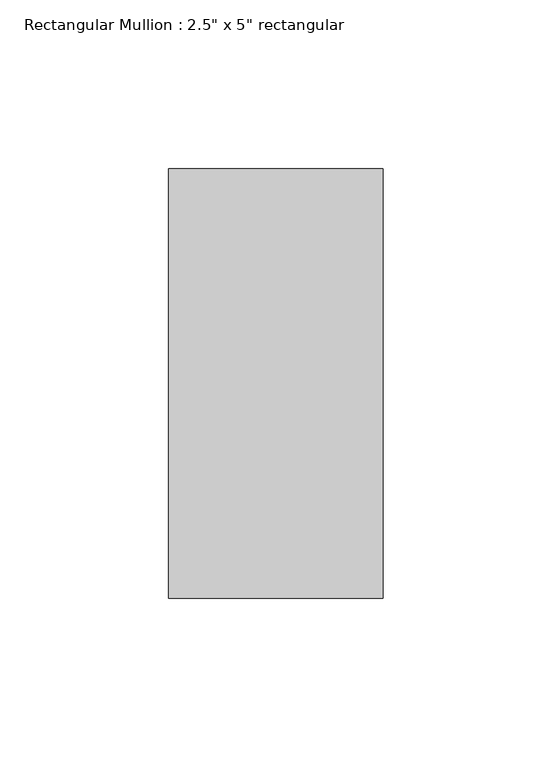
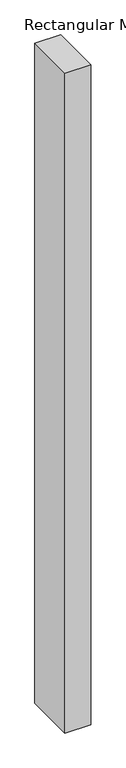
"""IFC4 building model written with IfcOpenShell, lengths in millimetres: member geometry."""

from ifc_helpers import new_model, si_unit, frame, origin, place, context, project, spatial, polyline, outline, extrude, source, transform, mapped, element, save


def member_6c7e385d(model_context):
    return source(origin(), model_context, "Body", "SweptSolid", [
        extrude(outline(polyline([(31.75, 63.5), (31.75, -63.5), (-31.75, -63.5), (-31.75, 63.5), (31.75, 63.5)])), frame((0.0, 0.0, -1708.8911809), z_axis=(0.0, 0.0, 1.0), x_axis=(1.0, 0.0, 0.0)), (0.0, 0.0, 1.0), 1708.8911809),
    ])


if __name__ == "__main__":
    model = new_model("IFC4")
    model_context = context("Model", 3, world=origin())
    ifc_project = project(units=[si_unit("LENGTHUNIT", "METRE", prefix="MILLI")], contexts=[model_context])
    site = spatial("IfcSite", under=ifc_project)
    building = spatial("IfcBuilding", under=site)
    placement = place(None, origin())
    member_shape = member_6c7e385d(model_context)
    element("IfcMember", 1, ObjectType="Rectangular Mullion : 2.5\" x 5\" rectangular", at=placement, inside=building, context=model_context, shape_type="MappedRepresentation", body=[
        mapped(member_shape, transform((0.0, 0.0, 0.0), x_axis=(1.0, 0.0, 0.0), y_axis=(0.0, 1.0, 0.0), z_axis=(0.0, 0.0, 1.0))),
    ])
    save(model, "model.ifc")

# Revit data of these elements
# Type "Rectangular Mullion : 2.5\" x 5\" rectangular"
#   built-in parameter 1007304 = 0.416667 (stored number, unit not read)
#   built-in parameter 1007301 = 0.104167 (stored number, unit not read)
#   built-in parameter 1007300 = 0.104167 (stored number, unit not read)
# Element 1 (IfcMember, "Rectangular Mullion : 2.5\" x 5\" rectangular")
#   Materials on its faces: "Aluminum"
# Materials
#   "Aluminum": class "Metal", colour RGB 247 247 247, transparency 0, Description = "Aluminum 6061", Cost = 0
